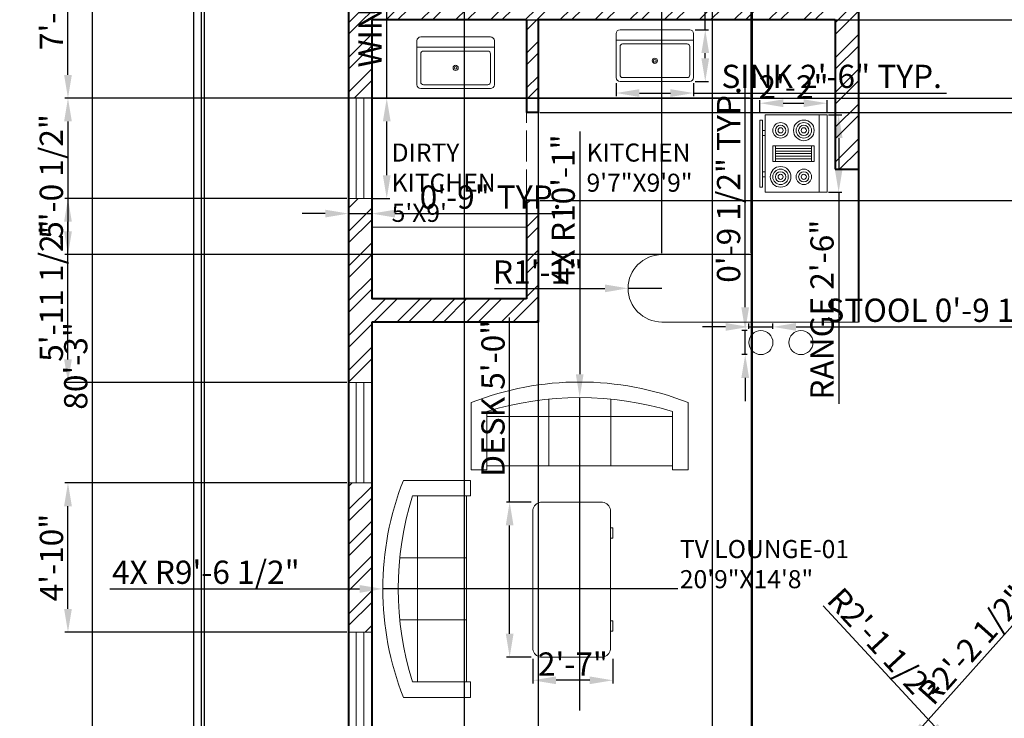
# Model space of a CAD drawing. Units: inches. Extents: x 3815 to 4442, y 1449 to 2534.
# Tile 3 of 5: x 3824 to 4205, y 1850 to 2120. Entities that reach past the tile are written whole.
import ezdxf

# ---------------------------------------------------------------- set-up
doc = ezdxf.new("R2010")
doc.units = ezdxf.units.IN
doc.linetypes.add('ACAD_ISO02W100', pattern=[15, 12, -3])
for name, color, linetype, lineweight in [('A-ANNO-DIMS', 2, 'Continuous', 18), ('A-AREA-IDEN', 7, 'Continuous', 20), ('A-EQPM', 8, 'Continuous', 18), ('A-FLOR-FIXD', 9, 'Continuous', 20), ('A-FLOR-FIXT', 8, 'Continuous', 18), ('A-FURN', 8, 'Continuous', 18), ('A-GLAZ', 4, 'Continuous', 20), ('A-WALL', 7, 'Continuous', 40), ('A-WALL-OVHD', 8, 'ACAD_ISO02W100', 18), ('A-WALL-PATT', 8, 'Continuous', 13), ('C-PROP', 7, 'Continuous', 30), ('L-PLNT-PATT', 9, 'Continuous', 13)]:
    doc.layers.add(name, color=color, linetype=linetype, lineweight=lineweight)
doc.styles.get("Standard").update_dxf_attribs({"font": 'arial.ttf'})
doc.dimstyles.new('ISO-25', dxfattribs={"dimtxt": 9, "dimasz": 9, "dimexe": 1.25, "dimexo": 0.625, "dimtad": 1, "dimdec": 1, "dimrnd": 9, "dimlunit": 3, "dimtxsty": 'Standard', "dimcen": 2.5, "dimadec": 0, "dimazin": 0, "dimtfac": 1, "dimtdec": 1, "dimtmove": 0, "dimatfit": 3, "dimfxl": 1, "dimarcsym": 0})

# ---------------------------------------------------------------- blocks, each defined once
blk = doc.blocks.new('*D2')
at = {"layer": 'A-ANNO-DIMS', "color": 0, "lineweight": -2, "transparency": 16777216}
for p, q in [((3890.5, 2466.24), (3850.63, 2466.24)), ((3851.88, 2457.24), (3851.88, 1515.24)), ((3890.5, 1506.24), (3850.63, 1506.24))]:
    blk.add_line(p, q, dxfattribs=at)
at = {"layer": 'A-ANNO-DIMS', "color": 0, "lineweight": 100, "transparency": 16777216}
for points in [[(3850.38, 2457.24), (3853.38, 2457.24), (3851.88, 2466.24)], [(3850.38, 1515.24), (3853.38, 1515.24), (3851.88, 1506.24)]]:
    blk.add_solid(points, dxfattribs=at)
at = {"layer": 'Defpoints', "color": 0, "lineweight": 100, "transparency": 16777216}
for p in [(3891.13, 2466.24), (3851.88, 1506.24), (3891.13, 1506.24)]:
    blk.add_point(p, dxfattribs=at)
at = {"layer": 'A-ANNO-DIMS', "color": 0, "transparency": 16777216, "insert": (3846.65, 1986.24), "char_height": 9, "attachment_point": 5, "rotation": 90}
blk.add_mtext('80\'-3"', dxfattribs=at)
blk = doc.blocks.new('Range-Oven - 30 in top')
for p, q in [((0, -3), (30, -3)), ((12, -6), (18, -6)), ((13, -20), (13, -6)), ((14, -6), (14, -20)), ((15, -20), (15, -6)), ((16, -6), (16, -20)), ((17, -20), (17, -6)), ((18, -20), (12, -20)), ((6, -24), (6, -25)), ((8, -25), (8, -24)), ((22, -25), (22, -24)), ((24, -24), (24, -25))]:
    blk.add_line(p, q)
for points in [[(0, -24), (0, 0), (30, 0), (30, -24)], [(12, -21), (12, -5), (18, -5), (18, -21)], [(2, -26), (2, -25), (28, -25), (28, -26)]]:
    blk.add_lwpolyline(points, close=True)
for centre, radius in [((6, -9), 4), ((6, -9), 3), ((6, -9), 2), ((24, -9), 3), ((24, -9), 2), ((6, -9), 1), ((24, -9), 1), ((6, -18), 3), ((24, -18), 4), ((24, -18), 3), ((6, -18), 2), ((6, -18), 1), ((24, -18), 2), ((24, -18), 1)]:
    blk.add_circle(centre, radius)
blk = doc.blocks.new('Sink-single - 30 in top')
blk.add_line((-15, -3.999996), (15, -3.999996))
for points in [[(-13.5, 0), (13.5, 0)], [(-15, -18.499996), (-15, -1.5)], [(15, -1.5), (15, -18.499996)], [(-13.5, -17.499996), (-13.5, -6.499996)], [(-12.5, -5.499996), (12.5, -5.499996)], [(13.5, -6.499996), (13.5, -17.499996)], [(12.5, -18.499996), (-12.5, -18.499996)], [(13.5, -19.999996), (-13.5, -19.999996)]]:
    blk.add_lwpolyline(points)
for radius in [1, 0.5]:
    blk.add_circle((0, -11.999996), radius)
for centre, radius, start, end in [((-13.5, -1.5), 1.5, 90, 180), ((13.5, -1.5), 1.5, 0, 90), ((-12.5, -6.499996), 1, 90, 180), ((12.5, -6.499996), 1, 0, 90), ((-13.5, -18.499996), 1.5, 180, 270), ((-12.5, -17.499996), 1, 180, 270), ((12.5, -17.499996), 1, 270, 0), ((13.5, -18.499996), 1.5, 270, 0)]:
    blk.add_arc(centre, radius, start, end)
blk = doc.blocks.new('Sofa - Roundback 7 ft.')
for p, q in [((-12.00002, -32.4421), (-12.00003, -6.5971)), ((11.99997, -32.4421), (11.99998, -6.5971)), ((-36.000027, -34), (-36.000027, -11.4696)), ((-35.999844, -13.3819), (35.9998, -13.3819)), ((35.99998, -34), (35.99998, -11.4696)), ((-36.000027, -32.4421), (35.99998, -32.4421))]:
    blk.add_line(p, q)
for points in [[(-36.000027, -34), (-42.000027, -34), (-42.000027, -8)], [(41.99998, -8), (41.99998, -34), (35.99998, -34)]]:
    blk.add_lwpolyline(points)
for centre, radius, start, end in [((0, -114.25), 114.25, 68.43141, 111.5686), ((-0.00001, -127.1968), 121.1968, 72.72033, 107.2797)]:
    blk.add_arc(centre, radius, start, end)
blk = doc.blocks.new('Desk - 30 x 60 in.')
for p, q in [((-26.999995, 0), (26.999995, 0)), ((-29.999995, -27), (-29.999995, -3)), ((29.999995, -3), (29.999995, -27)), ((26.999995, -30), (-26.999995, -30)), ((-20.000005, -30), (-20.000005, -31)), ((-16.000005, -31), (-16.000005, -30)), ((15.999995, -31), (15.999995, -30)), ((19.999995, -30), (19.999995, -31)), ((-20.000005, -31), (-16.000005, -31)), ((19.999995, -31), (15.999995, -31))]:
    blk.add_line(p, q)
for centre, start, end in [((-26.499995, -3.5), 98.1301, 171.8699), ((26.499995, -3.5), 8.130102, 81.8699), ((-26.499995, -26.5), 188.1301, 261.8699), ((26.499995, -26.5), 278.1301, 351.8699)]:
    blk.add_arc(centre, 3.535534, start, end)
blk = doc.blocks.new('WIN-W38-7_8-9IN')
for p, q in [((9, 38.85), (0, 38.85)), ((3, 38.85), (3, 0)), ((6, 38.85), (6, 0)), ((9, 0), (0, 0))]:
    blk.add_line(p, q)
blk = doc.blocks.new('STOOL-ROUND')
blk.add_circle((4.67, 4.67), 4.67)
blk = doc.blocks.new('*D26')
at = {"layer": 'A-ANNO-DIMS', "color": 0, "lineweight": -2, "transparency": 16777216}
for p, q in [((3965.95, 2089.9), (3965.95, 2214.04)), ((3960.75, 2089.9), (3967.2, 2089.9)), ((3965.95, 2060.05), (3965.95, 2080.9)), ((3960.75, 2051.05), (3967.2, 2051.05))]:
    blk.add_line(p, q, dxfattribs=at)
at = {"layer": 'A-ANNO-DIMS', "color": 0, "lineweight": 100, "transparency": 16777216}
for points in [[(3964.45, 2080.9), (3967.45, 2080.9), (3965.95, 2089.9)], [(3964.45, 2060.05), (3967.45, 2060.05), (3965.95, 2051.05)]]:
    blk.add_solid(points, dxfattribs=at)
at = {"layer": 'Defpoints', "color": 0, "lineweight": 100, "transparency": 16777216}
for p in [(3960.13, 2089.9), (3965.95, 2089.9), (3960.13, 2051.05)]:
    blk.add_point(p, dxfattribs=at)
at = {"layer": 'A-ANNO-DIMS', "color": 0, "transparency": 16777216, "insert": (3960.67, 2156.47), "char_height": 9, "attachment_point": 5, "rotation": 90}
blk.add_mtext('WINDOW 3\'-3" TYP.', dxfattribs=at)
blk = doc.blocks.new('*D27')
at = {"layer": 'A-ANNO-DIMS', "color": 0, "lineweight": -2, "transparency": 16777216}
for p, q in [((3951.13, 2050.42), (3951.13, 2043.97)), ((3960.13, 2050.42), (3960.13, 2043.97)), ((3942.13, 2045.22), (3933.13, 2045.22)), ((3951.13, 2045.22), (3960.13, 2045.22)), ((3969.13, 2045.22), (4034.24, 2045.22))]:
    blk.add_line(p, q, dxfattribs=at)
at = {"layer": 'A-ANNO-DIMS', "color": 0, "lineweight": 100, "transparency": 16777216}
for points in [[(3942.13, 2046.72), (3942.13, 2043.72), (3951.13, 2045.22)], [(3969.13, 2046.72), (3969.13, 2043.72), (3960.13, 2045.22)]]:
    blk.add_solid(points, dxfattribs=at)
at = {"layer": 'Defpoints', "color": 0, "lineweight": 100, "transparency": 16777216}
for p in [(3951.13, 2051.05), (3960.13, 2051.05), (3960.13, 2045.22)]:
    blk.add_point(p, dxfattribs=at)
at = {"layer": 'A-ANNO-DIMS', "color": 0, "transparency": 16777216, "insert": (4006.18, 2050.44), "char_height": 9, "attachment_point": 5}
blk.add_mtext('0\'-9" TYP.', dxfattribs=at)
blk = doc.blocks.new('*D30')
at = {"layer": 'A-ANNO-DIMS', "color": 0, "lineweight": -2, "transparency": 16777216}
for p, q in [((4054.82, 2095.78), (4054.82, 2090.66)), ((4084.82, 2095.78), (4084.82, 2090.66)), ((4063.82, 2091.91), (4075.82, 2091.91)), ((4084.82, 2091.91), (4182.73, 2091.91))]:
    blk.add_line(p, q, dxfattribs=at)
at = {"layer": 'A-ANNO-DIMS', "color": 0, "lineweight": 100, "transparency": 16777216}
for points in [[(4063.82, 2093.41), (4063.82, 2090.41), (4054.82, 2091.91)], [(4075.82, 2093.41), (4075.82, 2090.41), (4084.82, 2091.91)]]:
    blk.add_solid(points, dxfattribs=at)
at = {"layer": 'Defpoints', "color": 0, "lineweight": 100, "transparency": 16777216}
for p in [(4054.82, 2096.41), (4084.82, 2096.41), (4084.82, 2091.91)]:
    blk.add_point(p, dxfattribs=at)
at = {"layer": 'A-ANNO-DIMS', "color": 0, "transparency": 16777216, "insert": (4138.28, 2097.19), "char_height": 9, "attachment_point": 5}
blk.add_mtext('SINK 2\'-6" TYP.', dxfattribs=at)
blk = doc.blocks.new('*D31')
at = {"layer": 'A-ANNO-DIMS', "color": 0, "lineweight": -2, "transparency": 16777216}
for p, q in [((4089.32, 2116.41), (4089.32, 2180.67)), ((4085.45, 2116.41), (4090.57, 2116.41)), ((4089.32, 2105.41), (4089.32, 2107.41)), ((4085.45, 2096.41), (4090.57, 2096.41))]:
    blk.add_line(p, q, dxfattribs=at)
at = {"layer": 'A-ANNO-DIMS', "color": 0, "lineweight": 100, "transparency": 16777216}
for points in [[(4087.82, 2107.41), (4090.82, 2107.41), (4089.32, 2116.41)], [(4087.82, 2105.41), (4090.82, 2105.41), (4089.32, 2096.41)]]:
    blk.add_solid(points, dxfattribs=at)
at = {"layer": 'Defpoints', "color": 0, "lineweight": 100, "transparency": 16777216}
for p in [(4084.82, 2116.41), (4089.32, 2116.41), (4084.82, 2096.41)]:
    blk.add_point(p, dxfattribs=at)
at = {"layer": 'A-ANNO-DIMS', "color": 0, "transparency": 16777216, "insert": (4084.1, 2153.04), "char_height": 9, "attachment_point": 5, "rotation": 90}
blk.add_mtext('1\'-8" TYP.', dxfattribs=at)
blk = doc.blocks.new('*D40')
at = {"layer": 'A-ANNO-DIMS', "color": 0, "lineweight": -2, "transparency": 16777216}
for p, q in [((4106.2, 2000.57), (4106.2, 2002.6)), ((4115.53, 2000.57), (4115.53, 2002.6)), ((4097.2, 2001.35), (4088.2, 2001.35)), ((4106.2, 2001.35), (4115.53, 2001.35)), ((4124.53, 2001.35), (4256.68, 2001.35))]:
    blk.add_line(p, q, dxfattribs=at)
at = {"layer": 'A-ANNO-DIMS', "color": 0, "lineweight": 100, "transparency": 16777216}
for points in [[(4097.2, 2002.85), (4097.2, 1999.85), (4106.2, 2001.35)], [(4124.53, 2002.85), (4124.53, 1999.85), (4115.53, 2001.35)]]:
    blk.add_solid(points, dxfattribs=at)
at = {"layer": 'Defpoints', "color": 0, "lineweight": 100, "transparency": 16777216}
for p in [(4106.2, 1999.95), (4115.53, 2001.35), (4115.53, 1999.95)]:
    blk.add_point(p, dxfattribs=at)
at = {"layer": 'A-ANNO-DIMS', "color": 0, "transparency": 16777216, "insert": (4195.11, 2006.63), "char_height": 9, "attachment_point": 5}
blk.add_mtext('STOOL 0\'-9 1/2" TYP.', dxfattribs=at)
blk = doc.blocks.new('*D41')
at = {"layer": 'A-ANNO-DIMS', "color": 0, "lineweight": -2, "transparency": 16777216}
for p, q in [((4104.8, 2008.95), (4104.8, 2095.03)), ((4105.58, 1999.95), (4103.55, 1999.95)), ((4104.8, 1990.62), (4104.8, 1999.95)), ((4105.58, 1990.62), (4103.55, 1990.62)), ((4104.8, 1981.62), (4104.8, 1972.62))]:
    blk.add_line(p, q, dxfattribs=at)
at = {"layer": 'A-ANNO-DIMS', "color": 0, "lineweight": 100, "transparency": 16777216}
for points in [[(4103.3, 2008.95), (4106.3, 2008.95), (4104.8, 1999.95)], [(4103.3, 1981.62), (4106.3, 1981.62), (4104.8, 1990.62)]]:
    blk.add_solid(points, dxfattribs=at)
at = {"layer": 'Defpoints', "color": 0, "lineweight": 100, "transparency": 16777216}
for p in [(4104.8, 1999.95), (4106.2, 1999.95), (4106.2, 1990.62)]:
    blk.add_point(p, dxfattribs=at)
at = {"layer": 'A-ANNO-DIMS', "color": 0, "transparency": 16777216, "insert": (4099.52, 2056.49), "char_height": 9, "attachment_point": 5, "rotation": 90}
blk.add_mtext('0\'-9 1/2" TYP.', dxfattribs=at)
blk = doc.blocks.new('*D42')
at = {"layer": 'A-ANNO-DIMS', "color": 0, "lineweight": -2, "transparency": 16777216}
for p, q in [((4137.12, 2083.46), (4142.25, 2083.46)), ((4141, 2074.46), (4141, 2062.46)), ((4137.12, 2053.46), (4142.25, 2053.46)), ((4141, 2053.46), (4141, 1971.55))]:
    blk.add_line(p, q, dxfattribs=at)
at = {"layer": 'A-ANNO-DIMS', "color": 0, "lineweight": 100, "transparency": 16777216}
for points in [[(4139.5, 2074.46), (4142.5, 2074.46), (4141, 2083.46)], [(4139.5, 2062.46), (4142.5, 2062.46), (4141, 2053.46)]]:
    blk.add_solid(points, dxfattribs=at)
at = {"layer": 'Defpoints', "color": 0, "lineweight": 100, "transparency": 16777216}
for p in [(4136.5, 2083.46), (4136.5, 2053.46), (4141, 2053.46)]:
    blk.add_point(p, dxfattribs=at)
at = {"layer": 'A-ANNO-DIMS', "color": 0, "transparency": 16777216, "insert": (4135.72, 2008.01), "char_height": 9, "attachment_point": 5, "rotation": 90}
blk.add_mtext('RANGE 2\'-6"', dxfattribs=at)
blk = doc.blocks.new('*D43')
at = {"layer": 'A-ANNO-DIMS', "color": 0, "lineweight": -2, "transparency": 16777216}
for p, q in [((4110.5, 2084.09), (4110.5, 2089.21)), ((4119.5, 2087.96), (4127.5, 2087.96)), ((4136.5, 2084.09), (4136.5, 2089.21))]:
    blk.add_line(p, q, dxfattribs=at)
at = {"layer": 'A-ANNO-DIMS', "color": 0, "lineweight": 100, "transparency": 16777216}
for points in [[(4119.5, 2089.46), (4119.5, 2086.46), (4110.5, 2087.96)], [(4127.5, 2089.46), (4127.5, 2086.46), (4136.5, 2087.96)]]:
    blk.add_solid(points, dxfattribs=at)
at = {"layer": 'Defpoints', "color": 0, "lineweight": 100, "transparency": 16777216}
for p in [(4136.5, 2087.96), (4110.5, 2083.46), (4136.5, 2083.46)]:
    blk.add_point(p, dxfattribs=at)
at = {"layer": 'A-ANNO-DIMS', "color": 0, "transparency": 16777216, "insert": (4123.5, 2093.11), "char_height": 9, "attachment_point": 5}
blk.add_mtext('2\'-2"', dxfattribs=at)
blk = doc.blocks.new('*D44')
at = {"layer": 'A-ANNO-DIMS', "color": 0, "lineweight": -2, "transparency": 16777216}
for p, q in [((4013.56, 1933.49), (4013.56, 2004.94)), ((4021.93, 1933.49), (4012.31, 1933.49)), ((4013.56, 1882.49), (4013.56, 1924.49)), ((4021.93, 1873.49), (4012.31, 1873.49))]:
    blk.add_line(p, q, dxfattribs=at)
at = {"layer": 'A-ANNO-DIMS', "color": 0, "lineweight": 100, "transparency": 16777216}
for points in [[(4012.06, 1924.49), (4015.06, 1924.49), (4013.56, 1933.49)], [(4012.06, 1882.49), (4015.06, 1882.49), (4013.56, 1873.49)]]:
    blk.add_solid(points, dxfattribs=at)
at = {"layer": 'Defpoints', "color": 0, "lineweight": 100, "transparency": 16777216}
for p in [(4013.56, 1933.49), (4022.56, 1933.49), (4022.56, 1873.49)]:
    blk.add_point(p, dxfattribs=at)
at = {"layer": 'A-ANNO-DIMS', "color": 0, "transparency": 16777216, "insert": (4008.28, 1973.72), "char_height": 9, "attachment_point": 5, "rotation": 90}
blk.add_mtext('DESK 5\'-0"', dxfattribs=at)
blk = doc.blocks.new('*D45')
at = {"layer": 'A-ANNO-DIMS', "color": 0, "lineweight": -2, "transparency": 16777216}
for p, q in [((4022.56, 1872.86), (4022.56, 1863.24)), ((4053.56, 1872.86), (4053.56, 1863.24)), ((4044.56, 1864.49), (4031.56, 1864.49))]:
    blk.add_line(p, q, dxfattribs=at)
at = {"layer": 'A-ANNO-DIMS', "color": 0, "lineweight": 100, "transparency": 16777216}
for points in [[(4031.56, 1865.99), (4031.56, 1862.99), (4022.56, 1864.49)], [(4044.56, 1865.99), (4044.56, 1862.99), (4053.56, 1864.49)]]:
    blk.add_solid(points, dxfattribs=at)
at = {"layer": 'Defpoints', "color": 0, "lineweight": 100, "transparency": 16777216}
for p in [(4022.56, 1873.49), (4053.56, 1873.49), (4022.56, 1864.49)]:
    blk.add_point(p, dxfattribs=at)
at = {"layer": 'A-ANNO-DIMS', "color": 0, "transparency": 16777216, "insert": (4038.06, 1869.63), "char_height": 9, "attachment_point": 5}
blk.add_mtext('2\'-7"', dxfattribs=at)
blk = doc.blocks.new('*D54')
at = {"layer": 'A-ANNO-DIMS', "color": 0, "lineweight": -2, "transparency": 16777216}
for p, q in [((3996.13, 1823.37), (3996.13, 2516.14)), ((4005.13, 2514.89), (4083.13, 2514.89)), ((4092.13, 1823.37), (4092.13, 2516.14))]:
    blk.add_line(p, q, dxfattribs=at)
at = {"layer": 'A-ANNO-DIMS', "color": 0, "lineweight": 100, "transparency": 16777216}
for points in [[(4005.13, 2516.39), (4005.13, 2513.39), (3996.13, 2514.89)], [(4083.13, 2516.39), (4083.13, 2513.39), (4092.13, 2514.89)]]:
    blk.add_solid(points, dxfattribs=at)
at = {"layer": 'Defpoints', "color": 0, "lineweight": 100, "transparency": 16777216}
for p in [(4092.13, 2514.89), (3996.13, 1822.74), (4092.13, 1822.74)]:
    blk.add_point(p, dxfattribs=at)
at = {"layer": 'A-ANNO-DIMS', "color": 0, "transparency": 16777216, "insert": (4044.13, 2520.11), "char_height": 9, "attachment_point": 5}
blk.add_mtext('8\'-0"', dxfattribs=at)
blk = doc.blocks.new('*D56')
at = {"layer": 'A-ANNO-DIMS', "color": 0, "lineweight": -2, "transparency": 16777216}
for p, q in [((3950.5, 2175.52), (3841.23, 2175.52)), ((3842.48, 2098.9), (3842.48, 2166.52)), ((3950.5, 2089.9), (3841.23, 2089.9))]:
    blk.add_line(p, q, dxfattribs=at)
at = {"layer": 'A-ANNO-DIMS', "color": 0, "lineweight": 100, "transparency": 16777216}
for points in [[(3840.98, 2166.52), (3843.98, 2166.52), (3842.48, 2175.52)], [(3840.98, 2098.9), (3843.98, 2098.9), (3842.48, 2089.9)]]:
    blk.add_solid(points, dxfattribs=at)
at = {"layer": 'Defpoints', "color": 0, "lineweight": 100, "transparency": 16777216}
for p in [(3842.48, 2175.52), (3951.13, 2175.52), (3951.13, 2089.9)]:
    blk.add_point(p, dxfattribs=at)
at = {"layer": 'A-ANNO-DIMS', "color": 0, "transparency": 16777216, "insert": (3837.2, 2132.71), "char_height": 9, "attachment_point": 5, "rotation": 90}
blk.add_mtext('7\'-1 1/2"', dxfattribs=at)
blk = doc.blocks.new('*D57')
at = {"layer": 'A-ANNO-DIMS', "color": 0, "lineweight": -2, "transparency": 16777216}
for p, q in [((3950.5, 2051.05), (3841.23, 2051.05)), ((3842.48, 1988.78), (3842.48, 2042.05)), ((3950.5, 1979.78), (3841.23, 1979.78))]:
    blk.add_line(p, q, dxfattribs=at)
at = {"layer": 'A-ANNO-DIMS', "color": 0, "lineweight": 100, "transparency": 16777216}
for points in [[(3840.98, 2042.05), (3843.98, 2042.05), (3842.48, 2051.05)], [(3840.98, 1988.78), (3843.98, 1988.78), (3842.48, 1979.78)]]:
    blk.add_solid(points, dxfattribs=at)
at = {"layer": 'Defpoints', "color": 0, "lineweight": 100, "transparency": 16777216}
for p in [(3842.48, 2051.05), (3951.13, 2051.05), (3951.13, 1979.78)]:
    blk.add_point(p, dxfattribs=at)
at = {"layer": 'A-ANNO-DIMS', "color": 0, "transparency": 16777216, "insert": (3837.2, 2015.41), "char_height": 9, "attachment_point": 5, "rotation": 90}
blk.add_mtext('5\'-11 1/2"', dxfattribs=at)
blk = doc.blocks.new('*D58')
at = {"layer": 'A-ANNO-DIMS', "color": 0, "lineweight": -2, "transparency": 16777216}
for p, q in [((3950.5, 1940.92), (3841.23, 1940.92)), ((3842.48, 1892.13), (3842.48, 1931.92)), ((3950.5, 1883.13), (3841.23, 1883.13))]:
    blk.add_line(p, q, dxfattribs=at)
at = {"layer": 'A-ANNO-DIMS', "color": 0, "lineweight": 100, "transparency": 16777216}
for points in [[(3840.98, 1931.92), (3843.98, 1931.92), (3842.48, 1940.92)], [(3840.98, 1892.13), (3843.98, 1892.13), (3842.48, 1883.13)]]:
    blk.add_solid(points, dxfattribs=at)
at = {"layer": 'Defpoints', "color": 0, "lineweight": 100, "transparency": 16777216}
for p in [(3842.48, 1940.92), (3951.13, 1940.92), (3951.13, 1883.13)]:
    blk.add_point(p, dxfattribs=at)
at = {"layer": 'A-ANNO-DIMS', "color": 0, "transparency": 16777216, "insert": (3837.26, 1912.03), "char_height": 9, "attachment_point": 5, "rotation": 90}
blk.add_mtext('4\'-10"', dxfattribs=at)
blk = doc.blocks.new('*D63')
at = {"layer": 'A-ANNO-DIMS', "color": 0, "lineweight": -2, "transparency": 16777216}
for p, q in [((3895.33, 1506.87), (3895.33, 2516.14)), ((3904.33, 2514.89), (4098.56, 2514.89)), ((4107.56, 1506.87), (4107.56, 2516.14))]:
    blk.add_line(p, q, dxfattribs=at)
at = {"layer": 'A-ANNO-DIMS', "color": 0, "lineweight": 100, "transparency": 16777216}
for points in [[(3904.33, 2516.39), (3904.33, 2513.39), (3895.33, 2514.89)], [(4098.56, 2516.39), (4098.56, 2513.39), (4107.56, 2514.89)]]:
    blk.add_solid(points, dxfattribs=at)
at = {"layer": 'Defpoints', "color": 0, "lineweight": 100, "transparency": 16777216}
for p in [(4107.56, 2514.89), (3895.33, 1506.24), (4107.56, 1506.24)]:
    blk.add_point(p, dxfattribs=at)
at = {"layer": 'A-ANNO-DIMS', "color": 0, "transparency": 16777216, "insert": (4001.45, 2520.11), "char_height": 9, "attachment_point": 5}
blk.add_mtext('17\'-8"', dxfattribs=at)
blk = doc.blocks.new('*D66')
at = {"layer": 'A-ANNO-DIMS', "color": 0, "lineweight": -2, "transparency": 16777216}
for p, q in [((4024.63, 2089.28), (4024.63, 1456.34)), ((4107.04, 2089.28), (4107.04, 1456.34)), ((4033.63, 1457.59), (4098.04, 1457.59))]:
    blk.add_line(p, q, dxfattribs=at)
at = {"layer": 'A-ANNO-DIMS', "color": 0, "lineweight": 100, "transparency": 16777216}
for points in [[(4033.63, 1459.09), (4033.63, 1456.09), (4024.63, 1457.59)], [(4098.04, 1459.09), (4098.04, 1456.09), (4107.04, 1457.59)]]:
    blk.add_solid(points, dxfattribs=at)
at = {"layer": 'Defpoints', "color": 0, "lineweight": 100, "transparency": 16777216}
for p in [(4024.63, 2089.9), (4107.04, 2089.9), (4107.04, 1457.59)]:
    blk.add_point(p, dxfattribs=at)
at = {"layer": 'A-ANNO-DIMS', "color": 0, "transparency": 16777216, "insert": (4065.83, 1462.87), "char_height": 9, "attachment_point": 5}
blk.add_mtext('6\'-10 1/2"', dxfattribs=at)
blk = doc.blocks.new('*D67')
at = {"layer": 'A-ANNO-DIMS', "color": 0, "lineweight": -2, "transparency": 16777216}
for p, q in [((4419.78, 2120.24), (4419.78, 2175.54)), ((3960.75, 2120.24), (4421.03, 2120.24)), ((4419.78, 2098.9), (4419.78, 2111.24)), ((3960.75, 2089.9), (4421.03, 2089.9))]:
    blk.add_line(p, q, dxfattribs=at)
at = {"layer": 'A-ANNO-DIMS', "color": 0, "lineweight": 100, "transparency": 16777216}
for points in [[(4418.28, 2111.24), (4421.28, 2111.24), (4419.78, 2120.24)], [(4418.28, 2098.9), (4421.28, 2098.9), (4419.78, 2089.9)]]:
    blk.add_solid(points, dxfattribs=at)
at = {"layer": 'Defpoints', "color": 0, "lineweight": 100, "transparency": 16777216}
for p in [(3960.13, 2120.24), (4419.78, 2120.24), (3960.13, 2089.9)]:
    blk.add_point(p, dxfattribs=at)
at = {"layer": 'A-ANNO-DIMS', "color": 0, "transparency": 16777216, "insert": (4414.5, 2152.39), "char_height": 9, "attachment_point": 5, "rotation": 90}
blk.add_mtext('2\'-6 1/2"', dxfattribs=at)
blk = doc.blocks.new('*D68')
at = {"layer": 'A-ANNO-DIMS', "color": 0, "lineweight": -2, "transparency": 16777216}
for p, q in [((4025.25, 2084.42), (4421.03, 2084.42)), ((4419.78, 2059.34), (4419.78, 2075.42)), ((4025.25, 2050.34), (4421.03, 2050.34))]:
    blk.add_line(p, q, dxfattribs=at)
at = {"layer": 'A-ANNO-DIMS', "color": 0, "lineweight": 100, "transparency": 16777216}
for points in [[(4418.28, 2075.42), (4421.28, 2075.42), (4419.78, 2084.42)], [(4418.28, 2059.34), (4421.28, 2059.34), (4419.78, 2050.34)]]:
    blk.add_solid(points, dxfattribs=at)
at = {"layer": 'Defpoints', "color": 0, "lineweight": 100, "transparency": 16777216}
for p in [(4024.63, 2084.42), (4419.78, 2084.42), (4024.63, 2050.34)]:
    blk.add_point(p, dxfattribs=at)
at = {"layer": 'A-ANNO-DIMS', "color": 0, "transparency": 16777216, "insert": (4414.56, 2067.38), "char_height": 9, "attachment_point": 5, "rotation": 90}
blk.add_mtext('2\'-10"', dxfattribs=at)
blk = doc.blocks.new('*D72')
at = {"layer": 'A-ANNO-DIMS', "color": 0, "lineweight": -2, "transparency": 16777216}
for p, q in [((4106.42, 2089.9), (3841.23, 2089.9)), ((3842.48, 2080.9), (3842.48, 2038.32)), ((4106.42, 2029.32), (3841.23, 2029.32))]:
    blk.add_line(p, q, dxfattribs=at)
at = {"layer": 'A-ANNO-DIMS', "color": 0, "lineweight": 100, "transparency": 16777216}
for points in [[(3840.98, 2080.9), (3843.98, 2080.9), (3842.48, 2089.9)], [(3840.98, 2038.32), (3843.98, 2038.32), (3842.48, 2029.32)]]:
    blk.add_solid(points, dxfattribs=at)
at = {"layer": 'Defpoints', "color": 0, "lineweight": 100, "transparency": 16777216}
for p in [(4107.04, 2089.9), (3842.48, 2029.32), (4107.04, 2029.32)]:
    blk.add_point(p, dxfattribs=at)
at = {"layer": 'A-ANNO-DIMS', "color": 0, "transparency": 16777216, "insert": (3837.2, 2059.61), "char_height": 9, "attachment_point": 5, "rotation": 90}
blk.add_mtext('5\'-0 1/2"', dxfattribs=at)
blk = doc.blocks.new('*D73')
at = {"layer": 'A-ANNO-DIMS', "color": 0, "lineweight": -2, "transparency": 16777216}
for p, q in [((4072.48, 2029.94), (4072.48, 2516.14)), ((4081.48, 2514.89), (4098.04, 2514.89)), ((4107.04, 2029.94), (4107.04, 2516.14)), ((4107.04, 2514.89), (4169.33, 2514.89))]:
    blk.add_line(p, q, dxfattribs=at)
at = {"layer": 'A-ANNO-DIMS', "color": 0, "lineweight": 100, "transparency": 16777216}
for points in [[(4081.48, 2516.39), (4081.48, 2513.39), (4072.48, 2514.89)], [(4098.04, 2516.39), (4098.04, 2513.39), (4107.04, 2514.89)]]:
    blk.add_solid(points, dxfattribs=at)
at = {"layer": 'Defpoints', "color": 0, "lineweight": 100, "transparency": 16777216}
for p in [(4107.04, 2514.89), (4072.48, 2029.32), (4107.04, 2029.32)]:
    blk.add_point(p, dxfattribs=at)
at = {"layer": 'A-ANNO-DIMS', "color": 0, "transparency": 16777216, "insert": (4142.69, 2520.17), "char_height": 9, "attachment_point": 5}
blk.add_mtext('2\'-10 1/2"', dxfattribs=at)
blk = doc.blocks.new('*D78')
at = {"layer": 'A-ANNO-DIMS', "color": 0, "lineweight": -2, "transparency": 16777216}
for p, q in [((4007.66, 2016.28), (4050.45, 2016.28)), ((4072.48, 2016.28), (4059.45, 2016.28))]:
    blk.add_line(p, q, dxfattribs=at)
at = {"layer": 'A-ANNO-DIMS', "color": 0, "lineweight": 100, "transparency": 16777216}
blk.add_solid([(4050.45, 2017.78), (4050.45, 2014.78), (4059.45, 2016.28)], dxfattribs=at)
at = {"layer": 'Defpoints', "color": 0, "lineweight": 100, "transparency": 16777216}
for p in [(4059.45, 2016.28), (4072.48, 2016.28)]:
    blk.add_point(p, dxfattribs=at)
at = {"layer": 'A-ANNO-DIMS', "color": 0, "transparency": 16777216, "insert": (4024.55, 2021.42), "char_height": 9, "attachment_point": 5, "rotation": 359.9982}
blk.add_mtext('R1\'-1"', dxfattribs=at)
blk = doc.blocks.new('*D90')
at = {"layer": 'A-ANNO-DIMS', "color": 0, "lineweight": -2, "transparency": 16777216}
for p, q in [((4215.97, 1894.31), (4173.53, 1846.73)), ((4149.88, 1820.22), (4167.53, 1840.01))]:
    blk.add_line(p, q, dxfattribs=at)
at = {"layer": 'A-ANNO-DIMS', "color": 0, "lineweight": 100, "transparency": 16777216}
blk.add_solid([(4172.41, 1847.73), (4174.65, 1845.73), (4167.53, 1840.01)], dxfattribs=at)
at = {"layer": 'Defpoints', "color": 0, "lineweight": 100, "transparency": 16777216}
for p in [(4167.53, 1840.01), (4149.88, 1820.22)]:
    blk.add_point(p, dxfattribs=at)
at = {"layer": 'A-ANNO-DIMS', "color": 0, "transparency": 16777216, "insert": (4193.8, 1877.39), "char_height": 9, "attachment_point": 5, "rotation": 48.2637}
blk.add_mtext('R2\'-2 1/2"', dxfattribs=at)
blk = doc.blocks.new('*D91')
at = {"layer": 'A-ANNO-DIMS', "color": 0, "lineweight": -2, "transparency": 16777216}
for p, q in [((4134.94, 1893.34), (4178.27, 1846.57)), ((4201.68, 1821.3), (4184.39, 1839.97))]:
    blk.add_line(p, q, dxfattribs=at)
at = {"layer": 'A-ANNO-DIMS', "color": 0, "lineweight": 100, "transparency": 16777216}
blk.add_solid([(4179.37, 1847.59), (4177.17, 1845.55), (4184.39, 1839.97)], dxfattribs=at)
at = {"layer": 'Defpoints', "color": 0, "lineweight": 100, "transparency": 16777216}
for p in [(4184.39, 1839.97), (4201.68, 1821.3)]:
    blk.add_point(p, dxfattribs=at)
at = {"layer": 'A-ANNO-DIMS', "color": 0, "transparency": 16777216, "insert": (4157.42, 1876.84), "char_height": 9, "attachment_point": 5, "rotation": 312.817}
blk.add_mtext('R2\'-1 1/2"', dxfattribs=at)
blk = doc.blocks.new('*D92')
at = {"layer": 'A-ANNO-DIMS', "color": 0, "lineweight": -2, "transparency": 16777216}
for p, q in [((4040.69, 2076.97), (4040.69, 1983.01)), ((4040.69, 1852.81), (4040.69, 1974.01))]:
    blk.add_line(p, q, dxfattribs=at)
at = {"layer": 'A-ANNO-DIMS', "color": 0, "lineweight": 100, "transparency": 16777216}
blk.add_solid([(4039.19, 1983.01), (4042.19, 1983.01), (4040.69, 1974.01)], dxfattribs=at)
at = {"layer": 'Defpoints', "color": 0, "lineweight": 100, "transparency": 16777216}
for p in [(4040.69, 1974.01), (4040.69, 1852.81)]:
    blk.add_point(p, dxfattribs=at)
at = {"layer": 'A-ANNO-DIMS', "color": 0, "transparency": 16777216, "insert": (4035.47, 2046.73), "char_height": 9, "attachment_point": 5, "rotation": 89.9998}
blk.add_mtext('4X R10\'-1"', dxfattribs=at)
blk = doc.blocks.new('*D93')
at = {"layer": 'A-ANNO-DIMS', "color": 0, "lineweight": -2, "transparency": 16777216}
for p, q in [((3858.64, 1899.89), (3955.42, 1899.89)), ((4078.67, 1899.89), (3964.42, 1899.89))]:
    blk.add_line(p, q, dxfattribs=at)
at = {"layer": 'A-ANNO-DIMS', "color": 0, "lineweight": 100, "transparency": 16777216}
blk.add_solid([(3955.42, 1901.39), (3955.42, 1898.39), (3964.42, 1899.89)], dxfattribs=at)
at = {"layer": 'Defpoints', "color": 0, "lineweight": 100, "transparency": 16777216}
for p in [(3964.42, 1899.89), (4078.67, 1899.89)]:
    blk.add_point(p, dxfattribs=at)
at = {"layer": 'A-ANNO-DIMS', "color": 0, "transparency": 16777216, "insert": (3895.87, 1905.17), "char_height": 9, "attachment_point": 5, "rotation": 0.0002}
blk.add_mtext('4X R9\'-6 1/2"', dxfattribs=at)

msp = doc.modelspace()

# ---------------------------------------------------------------- hatches: boundary and pattern name
at = {"layer": 'A-WALL-PATT'}
h = msp.add_hatch(dxfattribs=at)
h.set_pattern_fill('ANSI32', color=256)
h.paths.add_polyline_path([(4156.29, 2346.24), (3989.15, 2346.24), (3989.15, 2337.24), (4044.13, 2337.24), (4044.13, 2305.59, -0.025534), (4046.38, 2305.51), (4048.63, 2305.51), (4048.63, 2337.24), (4139.63, 2337.24), (4139.63, 2277.24), (4112.45, 2277.24), (4112.45, 2272.74), (4139.63, 2272.74), (4139.63, 2180.66), (4148.63, 2180.66), (4148.63, 2184.24), (4208.63, 2184.24), (4208.63, 2180.66), (4213.13, 2180.66), (4213.13, 2209.79), (4208.63, 2209.79), (4208.63, 2188.74), (4148.63, 2188.74), (4148.63, 2254.74), (4185.97, 2254.74), (4185.97, 2259.24), (4148.63, 2259.24), (4148.63, 2337.24), (4156.29, 2337.24)])
h.paths.add_polyline_path([(4251.85, 2346.24), (4180.29, 2346.24), (4180.29, 2337.24), (4208.63, 2337.24), (4208.63, 2259.24), (4205.62, 2259.24), (4205.62, 2254.74), (4208.63, 2254.74), (4208.63, 2245.05), (4213.13, 2245.05), (4213.13, 2337.24), (4251.85, 2337.24)])
h.paths.add_polyline_path([(4371.13, 2346.24), (4311.85, 2346.24), (4311.85, 2337.24), (4362.13, 2337.24), (4362.13, 2129.24), (4213.13, 2129.24), (4213.13, 2137.97), (4208.63, 2137.97), (4208.63, 2111.87), (4217.63, 2111.87), (4217.63, 2120.24), (4362.13, 2120.24), (4362.13, 1643.24), (4318.71, 1643.24), (4318.71, 1634.24), (4371.13, 1634.24)])
h.paths.add_polyline_path([(3960.13, 2175.52), (3951.13, 2175.52), (3951.13, 2089.9), (3960.13, 2089.9), (3960.13, 2120.24), (4020.13, 2120.24), (4020.13, 2084.42), (4024.63, 2084.42), (4024.63, 2120.24), (4139.63, 2120.24), (4139.63, 2062.37), (4148.63, 2062.37), (4148.63, 2137.97), (4139.63, 2137.97), (4139.63, 2129.24), (3960.13, 2129.24)])
h.paths.add_polyline_path([(3960.13, 2272.74), (4044.13, 2272.74), (4079.8, 2272.74), (4079.8, 2277.24), (4048.63, 2277.24), (4048.63, 2282.04), (4044.13, 2282.04), (4044.13, 2277.24), (3960.13, 2277.24), (3960.13, 2337.24), (3965.15, 2337.24), (3965.15, 2346.24), (3951.13, 2346.24), (3951.13, 2235.52), (3960.13, 2235.52)])
h.paths.add_polyline_path([(4024.63, 2050.34), (4020.13, 2050.34), (4020.13, 2012.24), (3960.13, 2012.24), (3960.13, 2051.05), (3951.13, 2051.05), (3951.13, 1979.78), (3960.13, 1979.78), (3960.13, 2003.24), (4024.63, 2003.24)])
h.paths.add_polyline_path([(4217.63, 2072.24), (4208.63, 2072.24), (4208.63, 2015.24), (4362.13, 2015.24), (4362.13, 2024.24), (4217.63, 2024.24)], flags=17)
h.paths.add_polyline_path([(3960.13, 1940.92), (3951.13, 1940.92), (3951.13, 1883.13), (3960.13, 1883.13)])
h.paths.add_polyline_path([(3960.13, 1822.74), (4149.38, 1822.74), (4149.38, 1827.24), (3960.13, 1827.24), (3960.13, 1844.28), (3951.13, 1844.28), (3951.13, 1769.4), (3960.13, 1769.4)])
h.paths.add_polyline_path([(4362.13, 1827.24), (4326.89, 1827.24), (4326.89, 1818.24), (4362.13, 1818.24)], flags=17)
h.paths.add_polyline_path([(4244.38, 1827.24), (4208.63, 1827.24), (4203.18, 1827.24), (4203.18, 1822.74), (4208.63, 1822.74), (4208.63, 1812.3), (4217.63, 1812.3), (4217.63, 1818.24), (4244.38, 1818.24)])
h.paths.add_polyline_path([(4149.38, 1738.74), (4142.66, 1738.74), (4142.66, 1742.16), (4138.16, 1742.16), (4138.16, 1738.74), (4090.16, 1738.74), (4090.16, 1774.74), (4138.16, 1774.74), (4138.16, 1763.78), (4142.66, 1763.78), (4142.66, 1774.74), (4142.66, 1779.24), (4138.16, 1779.24), (4090.16, 1779.24), (4085.66, 1779.24), (4085.66, 1774.74), (4085.66, 1738.74), (3960.13, 1738.74), (3960.13, 1743.46), (3951.13, 1743.46), (3951.13, 1729.74), (4149.38, 1729.74)])
h.paths.add_polyline_path([(4136.7, 1703.49), (4136.7, 1729.74), (4127.7, 1729.74), (4127.7, 1703.49), (4127.7, 1701.02), (4181.38, 1655.79), (4183.63, 1655.79), (4208.63, 1655.79), (4208.63, 1664.79), (4183.63, 1664.79)])
h.paths.add_polyline_path([(4217.63, 1771.49), (4208.63, 1771.49), (4208.63, 1738.74), (4202.94, 1738.74), (4202.94, 1729.74), (4208.63, 1729.74), (4208.63, 1634.24), (4258.71, 1634.24), (4258.71, 1643.24), (4217.63, 1643.24)])
at = {"layer": 'L-PLNT-PATT'}
h = msp.add_hatch(dxfattribs=at)
h.set_pattern_fill('GOST_GLASS', color=256)
h.paths.add_polyline_path([(4368.13, 2463.24), (3894.13, 2463.24, -0.246049), (3960.13, 2346.24), (4368.13, 2346.24)])
h.paths.add_polyline_path([(4365.15, 1631.83), (4112.05, 1631.83), (4112.05, 1581.3), (4365.15, 1581.3)])
h.paths.add_polyline_path([(4365.15, 1581.3), (4112.05, 1581.3), (4112.05, 1511.54), (4365.15, 1511.54)])
h.paths.add_polyline_path([(4219.4, 1545.72), (4287.81, 1545.72), (4287.81, 1571.84), (4219.4, 1571.84)], flags=24)

# ---------------------------------------------------------------- linework, layer by layer
at = {"layer": 'A-FLOR-FIXD'}
for p, q in [((4020.13, 2089.9), (3960.13, 2089.9)), ((4024.63, 2089.9), (4107.04, 2089.9)), ((4107.04, 2089.9), (4107.04, 2029.32)), ((4020.13, 2039.99), (3960.13, 2039.99)), ((4107.04, 2029.32), (4072.48, 2029.32)), ((4148.63, 2003.24), (4072.48, 2003.24))]:
    msp.add_line(p, q, dxfattribs=at)
msp.add_arc((4072.48, 2016.28), 13.04, 90, 270, dxfattribs=at)
at = {"layer": 'A-WALL'}
for p, q in [((3951.13, 2346.24), (3951.13, 1729.74)), ((4148.63, 2137.97), (4148.63, 2003.24)), ((3960.13, 2120.24), (3960.13, 2012.24)), ((4020.13, 2120.24), (3960.13, 2120.24)), ((4020.13, 2120.24), (4020.13, 2084.42)), ((4024.63, 2120.24), (4024.63, 2084.42)), ((4139.63, 2120.24), (4024.63, 2120.24)), ((4139.63, 2120.24), (4139.63, 2062.37)), ((4024.63, 2084.42), (4020.13, 2084.42)), ((4139.63, 2062.37), (4148.63, 2062.37)), ((4024.63, 2050.34), (4020.13, 2050.34)), ((4020.13, 2050.34), (4020.13, 2012.24)), ((4024.63, 2050.34), (4024.63, 2003.24)), ((4020.13, 2012.24), (3960.13, 2012.24)), ((4024.63, 2003.24), (3960.13, 2003.24)), ((3960.13, 2003.24), (3960.13, 1827.24))]:
    msp.add_line(p, q, dxfattribs=at)
at = {"layer": 'A-WALL-OVHD'}
for p, q in [((4020.13, 2050.34), (4020.13, 2084.42)), ((4024.63, 2050.34), (4024.63, 2084.42))]:
    msp.add_line(p, q, dxfattribs=at)
at = {"layer": 'C-PROP'}
for p, q in [((3891.13, 2466.24), (3891.13, 1506.24)), ((3894.13, 2463.24), (3894.13, 1510.52))]:
    msp.add_line(p, q, dxfattribs=at)

# ---------------------------------------------------------------- block references
at = {"layer": 'A-EQPM', "rotation": 270}
msp.add_blockref('Range-Oven - 30 in top', (4136.5, 2083.46), dxfattribs=at)
at = {"layer": 'A-FLOR-FIXT'}
for p in [(3992.63, 2113.64), (4069.82, 2116.41)]:
    msp.add_blockref('Sink-single - 30 in top', p, dxfattribs=at)
at = {"layer": 'A-FURN'}
for name, p in [('STOOL-ROUND', (4106.2, 1990.62)), ('STOOL-ROUND', (4121.7, 1990.62)), ('Sofa - Roundback 7 ft.', (4040.69, 1980.01))]:
    msp.add_blockref(name, p, dxfattribs=at)
at = {"layer": 'A-FURN', "rotation": 90}
for name, p in [('Sofa - Roundback 7 ft.', (3964.42, 1899.89)), ('Desk - 30 x 60 in.', (4022.56, 1903.49))]:
    msp.add_blockref(name, p, dxfattribs=at)
at = {"layer": 'A-GLAZ'}
for p in [(3951.13, 2051.05), (3951.13, 1940.92), (3951.13, 1844.28)]:
    msp.add_blockref('WIN-W38-7_8-9IN', p, dxfattribs=at)

# ---------------------------------------------------------------- texts
at = {"layer": 'A-AREA-IDEN', "char_height": 7, "attachment_point": 1}
for s, width, insert in [("DIRTY\\PKITCHEN\\P5'X9'", 62.2181, (3967.86, 2072.36)), ('KITCHEN\\P9\'7"X9\'9"', 62.2181, (4043.34, 2072.36)), ('TV LOUNGE-01\\P20\'9"X14\'8"', 105.0101, (4079.48, 1918.82))]:
    msp.add_mtext_dynamic_manual_height_columns(s, width=width, gutter_width=12.5, heights=[0], dxfattribs=dict(at, insert=insert))

# ---------------------------------------------------------------- dimensions: what is measured, and where the dimension line sits
at = {"layer": 'A-ANNO-DIMS'}
for base, p1, p2, picture, middle in [((4107.04, 2514.89), (4072.48, 2029.32), (4107.04, 2029.32), '*D73', (4142.69, 2520.17)), ((4107.56, 2514.89), (3895.33, 1506.24), (4107.56, 1506.24), '*D63', (4001.45, 2520.11)), ((4092.13, 2514.89), (3996.13, 1822.74), (4092.13, 1822.74), '*D54', (4044.13, 2520.11)), ((4136.5, 2087.96), (4110.5, 2083.46), (4136.5, 2083.46), '*D43', (4123.5, 2093.11)), ((4107.04, 1457.59), (4024.63, 2089.9), (4107.04, 2089.9), '*D66', (4065.83, 1462.87))]:
    dim = msp.add_linear_dim(base=base, p1=p1, p2=p2, dimstyle='ISO-25', override={"dimdec": 1, "dimlfac": 1, "dimrnd": 0, "dimzin": 1, "dimdsep": 46, "dimlunit": 4, "dimfrac": 2}, dxfattribs=at)
    dim.commit()
    dim.dimension.update_dxf_attribs({"geometry": picture, "text_midpoint": middle})
for base, p1, p2, angle, override, picture, middle in [((3851.88, 1506.24), (3891.13, 2466.24), (3891.13, 1506.24), 90, {"dimclrd": 0, "dimclre": 0, "dimclrt": 0}, '*D2', (3846.65, 1986.24)), ((3842.48, 2175.52), (3951.13, 2089.9), (3951.13, 2175.52), 90, {"dimdec": 1, "dimlfac": 1, "dimrnd": 0, "dimzin": 1, "dimdsep": 46, "dimlunit": 4, "dimfrac": 2}, '*D56', (3837.2, 2132.71)), ((4419.78, 2120.24), (3960.13, 2089.9), (3960.13, 2120.24), 90, {"dimdec": 1, "dimlfac": 1, "dimrnd": 0, "dimzin": 1, "dimdsep": 46, "dimlunit": 4, "dimfrac": 2}, '*D67', (4414.5, 2152.39)), ((3842.48, 2029.32), (4107.04, 2089.9), (4107.04, 2029.32), 90, {"dimdec": 1, "dimlfac": 1, "dimrnd": 0, "dimzin": 1, "dimdsep": 46, "dimlunit": 4, "dimfrac": 2}, '*D72', (3837.2, 2059.61)), ((4419.78, 2084.42), (4024.63, 2050.34), (4024.63, 2084.42), 90, {"dimdec": 1, "dimlfac": 1, "dimrnd": 0, "dimzin": 1, "dimdsep": 46, "dimlunit": 4, "dimfrac": 2}, '*D68', (4414.56, 2067.38)), ((3842.48, 2051.05), (3951.13, 1979.78), (3951.13, 2051.05), 90, {"dimdec": 1, "dimlfac": 1, "dimrnd": 0, "dimzin": 1, "dimdsep": 46, "dimlunit": 4, "dimfrac": 2}, '*D57', (3837.2, 2015.41)), ((3842.48, 1940.92), (3951.13, 1883.13), (3951.13, 1940.92), 90, {"dimdec": 1, "dimlfac": 1, "dimrnd": 0, "dimzin": 1, "dimdsep": 46, "dimlunit": 4, "dimfrac": 2}, '*D58', (3837.26, 1912.03)), ((4022.56, 1864.49), (4053.56, 1873.49), (4022.56, 1873.49), 180, {"dimdec": 1, "dimlfac": 1, "dimrnd": 0, "dimzin": 1, "dimdsep": 46, "dimlunit": 4, "dimfrac": 2}, '*D45', (4038.06, 1869.63))]:
    dim = msp.add_linear_dim(base=base, p1=p1, p2=p2, angle=angle, dimstyle='ISO-25', override=override, dxfattribs=at)
    dim.commit()
    dim.dimension.update_dxf_attribs({"geometry": picture, "text_midpoint": middle})
for base, p1, p2, angle, text, picture, middle in [((3965.9546, 2089.9011), (3960.1265, 2051.0475), (3960.1265, 2089.9011), 90, 'WINDOW <> TYP.', '*D26', (3960.6699, 2156.4698)), ((4089.32, 2116.41), (4084.82, 2096.41), (4084.82, 2116.41), 90, '<> TYP.', '*D31', (4084.1, 2153.04)), ((4104.8, 1999.95), (4106.2, 1990.62), (4106.2, 1999.95), 90, '<> TYP.', '*D41', (4099.52, 2056.49)), ((4141, 2053.46), (4136.5, 2083.46), (4136.5, 2053.46), 270, 'RANGE <>', '*D42', (4135.72, 2008.01)), ((4013.56, 1933.49), (4022.56, 1873.49), (4022.56, 1933.49), 90, 'DESK <>', '*D44', (4008.28, 1973.72))]:
    dim = msp.add_linear_dim(base=base, p1=p1, p2=p2, angle=angle, text=text, dimstyle='ISO-25', override={"dimdec": 1, "dimlfac": 1, "dimrnd": 0, "dimzin": 1, "dimdsep": 46, "dimlunit": 4, "dimfrac": 2}, dxfattribs=at)
    dim.commit()
    dim.dimension.update_dxf_attribs({"geometry": picture, "text_midpoint": middle})
for base, p1, p2, text, picture, middle in [((4084.82, 2091.91), (4054.82, 2096.41), (4084.82, 2096.41), 'SINK <> TYP.', '*D30', (4138.28, 2097.19)), ((3960.13, 2045.22), (3951.13, 2051.05), (3960.13, 2051.05), '<> TYP.', '*D27', (4006.18, 2050.44)), ((4115.53, 2001.35), (4106.2, 1999.95), (4115.53, 1999.95), 'STOOL <> TYP.', '*D40', (4195.11, 2006.63))]:
    dim = msp.add_linear_dim(base=base, p1=p1, p2=p2, text=text, dimstyle='ISO-25', override={"dimdec": 1, "dimlfac": 1, "dimrnd": 0, "dimzin": 1, "dimdsep": 46, "dimlunit": 4, "dimfrac": 2}, dxfattribs=at)
    dim.commit()
    dim.dimension.update_dxf_attribs({"geometry": picture, "text_midpoint": middle})
for center, mpoint, picture, middle in [((4040.69, 1852.81), (4040.69, 1974.01), '*D92', (4040.69, 2046.73)), ((4078.671929, 1899.887464), (3964.421929, 1899.887), '*D93', (3895.871929, 1899.8867216))]:
    dim = msp.add_radius_dim(center=center, mpoint=mpoint, text='4X <>', dimstyle='ISO-25', override={"dimdec": 1, "dimlfac": 1, "dimrnd": 0, "dimzin": 1, "dimdsep": 46, "dimlunit": 4, "dimfrac": 2}, dxfattribs=at)
    dim.commit()
    dim.dimension.update_dxf_attribs({"geometry": picture, "text_midpoint": middle, "dimtype": 164})
for center, mpoint, picture, middle in [((4072.48, 2016.28), (4059.45, 2016.28), '*D78', (4024.55, 2021.42)), ((4201.68, 1821.3), (4184.39, 1839.97), '*D91', (4157.42, 1876.84)), ((4149.88, 1820.22), (4167.53, 1840.01), '*D90', (4193.8, 1877.39))]:
    dim = msp.add_radius_dim(center=center, mpoint=mpoint, dimstyle='ISO-25', override={"dimdec": 1, "dimlfac": 1, "dimrnd": 0, "dimzin": 1, "dimdsep": 46, "dimlunit": 4, "dimfrac": 2}, dxfattribs=at)
    dim.commit()
    dim.dimension.update_dxf_attribs({"geometry": picture, "text_midpoint": middle})

doc.saveas('drawing.dxf')
